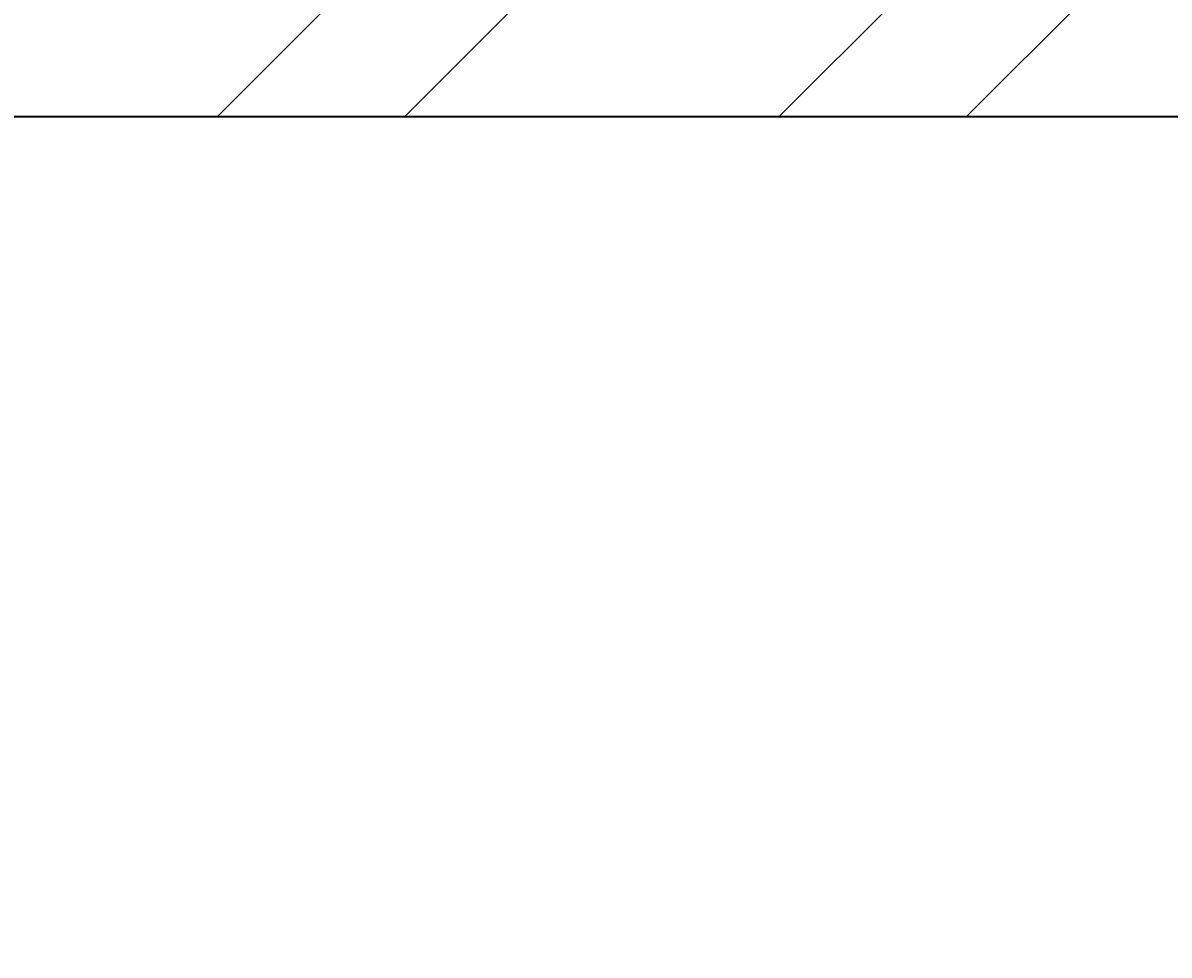
# Model space of a CAD drawing. Units: inches. Extents: x 1962 to 2771, y 1245 to 2660.
# Tile 70 of 114: x 2523 to 2551, y 2158 to 2180. Entities that reach past the tile are written whole.
import ezdxf

# ---------------------------------------------------------------- set-up
doc = ezdxf.new("R2010")
doc.units = ezdxf.units.IN
for name, color, linetype, lineweight in [('A-ANNO-DIMS', 2, 'Continuous', 18), ('A-WALL', 7, 'Continuous', 35), ('A-WALL-PATT', 252, 'Continuous', 13)]:
    doc.layers.add(name, color=color, linetype=linetype, lineweight=lineweight)
doc.styles.get("Standard").update_dxf_attribs({"font": 'arial.ttf'})
doc.dimstyles.get("Standard").update_dxf_attribs({"dimtxt": 0.18, "dimasz": 0.18, "dimexe": 0.18, "dimexo": 0.0625, "dimgap": 0.09, "dimtad": 0, "dimtih": 1, "dimtoh": 1, "dimdec": 4, "dimzin": 0, "dimdsep": 46, "dimtxsty": 'Standard', "dimcen": 0.09, "dimadec": 0, "dimazin": 0, "dimtfac": 1, "dimtdec": 4, "dimtofl": 0, "dimtmove": 0, "dimatfit": 3, "dimfxl": 1, "dimtolj": 1, "dimtzin": 0, "dimarcsym": 0})

# ---------------------------------------------------------------- blocks, each defined once
blk = doc.blocks.new('*D40')
at = {"layer": 'A-ANNO-DIMS', "color": 0, "lineweight": -2, "transparency": 16777216}
for p, q in [((2072.02, 2033.906), (2072.02, 2583.474)), ((2660.807, 2524.406), (2660.807, 2583.474)), ((2072.2, 2583.294), (2366.02, 2583.294)), ((2660.627, 2583.294), (2366.808, 2583.294))]:
    blk.add_line(p, q, dxfattribs=at)
at = {"layer": 'A-ANNO-DIMS', "color": 0, "transparency": 16777216}
for points in [[(2072.2, 2583.324), (2072.2, 2583.264), (2072.02, 2583.294)], [(2660.627, 2583.324), (2660.627, 2583.264), (2660.807, 2583.294)]]:
    blk.add_solid(points, dxfattribs=at)
at = {"layer": 'Defpoints', "color": 0, "transparency": 16777216}
for p in [(2660.807, 2583.294), (2660.807, 2524.344), (2072.02, 2033.844)]:
    blk.add_point(p, dxfattribs=at)
at = {"layer": 'A-ANNO-DIMS', "color": 0, "transparency": 16777216, "insert": (2366.414, 2583.294), "char_height": 0.18, "attachment_point": 5}
blk.add_mtext('\\A1;588.8', dxfattribs=at)

msp = doc.modelspace()

# ---------------------------------------------------------------- hatches: boundary and pattern name
at = {"layer": 'A-WALL-PATT'}
h = msp.add_hatch(dxfattribs=at)
h.set_pattern_fill('ANSI32', color=256)
h.paths.add_polyline_path([(2090.8074, 2467.3437), (2141.6481, 2467.3437), (2141.6481, 2469.5937), (2141.6481, 2471.8437), (2086.3074, 2471.8437), (2086.3074, 2422.5333), (2090.8074, 2422.5333)])
h.paths.add_polyline_path([(2282.7664, 2471.8437), (2204.8982, 2471.8437), (2204.8982, 2467.3437), (2234.8074, 2467.3437), (2234.8074, 2311.3437), (2228.7492, 2311.3437), (2228.7492, 2306.8437), (2234.8074, 2306.8437), (2331.9227, 2306.8437), (2331.9227, 2309.0937), (2331.9227, 2311.3437), (2239.3074, 2311.3437), (2239.3074, 2467.3437), (2282.7664, 2467.3437), (2282.7664, 2469.5937)])
h.paths.add_polyline_path([(2471.4531, 2519.8437), (2552.011, 2519.8437), (2564.3996, 2519.8437), (2564.3996, 2511.1389), (2568.8996, 2511.1389), (2568.8996, 2524.3437), (2466.9531, 2524.3437), (2466.9531, 2471.8437), (2450.0749, 2471.8437), (2446.4672, 2471.8437), (2446.4672, 2467.3437), (2450.0749, 2467.3437), (2475.9988, 2467.3437), (2475.9988, 2469.5937), (2475.9988, 2471.8437), (2471.4531, 2471.8437)])
h.paths.add_polyline_path([(2575.2231, 2469.5937), (2575.2231, 2471.8437), (2568.8996, 2471.8437), (2568.8996, 2487.1389), (2564.3996, 2487.1389), (2564.3996, 2471.8437), (2556.511, 2471.8437), (2499.2904, 2471.8437), (2499.2904, 2467.3437), (2507.8074, 2467.3437), (2507.8074, 2311.3437), (2414.863, 2311.3437), (2414.863, 2306.8437), (2512.3074, 2306.8437), (2517.0114, 2306.8437), (2517.0114, 2309.0937), (2517.0114, 2311.3437), (2512.3074, 2311.3437), (2512.3074, 2467.3437), (2575.2231, 2467.3437)])
h.paths.add_polyline_path([(2660.8074, 2471.8437), (2600.9602, 2471.8437), (2600.9602, 2467.3437), (2656.3074, 2467.3437), (2656.3074, 2432.5704), (2660.8074, 2432.5704)])
h.paths.add_polyline_path([(2660.8074, 2372.5704), (2656.3074, 2372.5704), (2656.3074, 2311.3437), (2600.276, 2311.3437), (2600.276, 2309.0937), (2600.276, 2306.8437), (2656.3074, 2306.8437), (2656.3074, 2296.2593), (2660.8074, 2296.2593)])
h.paths.add_polyline_path([(2572.3074, 2306.8437), (2577.1385, 2306.8437), (2577.1385, 2311.3437), (2551.082, 2311.3437), (2551.082, 2306.8437), (2567.8074, 2306.8437), (2567.8074, 2258.8437), (2540.0574, 2258.8437), (2540.0574, 2256.5937), (2540.0574, 2254.3437), (2567.8074, 2254.3437), (2656.3074, 2254.3437), (2656.3074, 2236.9085), (2660.8074, 2236.9085), (2660.8074, 2272.2593), (2656.3074, 2272.2593), (2656.3074, 2258.8437), (2572.3074, 2258.8437)])
h.paths.add_polyline_path([(2512.3074, 2254.3437), (2518.8716, 2254.3437), (2518.8716, 2256.5937), (2518.8716, 2258.8437), (2507.8074, 2258.8437), (2507.8074, 2177.8437), (2567.8074, 2177.8437), (2567.8074, 2172.9628), (2572.3074, 2172.9628), (2572.3074, 2177.8437), (2656.3074, 2177.8437), (2656.3074, 2166.4846), (2660.8074, 2166.4846), (2660.8074, 2200.9085), (2656.3074, 2200.9085), (2656.3074, 2182.3437), (2512.3074, 2182.3437)])
h.paths.add_polyline_path([(2656.3074, 2129.8437), (2572.3074, 2129.8437), (2572.3074, 2150.3044), (2570.0574, 2150.3044), (2567.8074, 2150.3044), (2567.8074, 2129.8437), (2507.8074, 2129.8437), (2507.8074, 2116.3027), (2510.0574, 2116.3027), (2512.3074, 2116.3027), (2512.3074, 2125.3437), (2567.8074, 2125.3437), (2572.3074, 2125.3437), (2656.3074, 2125.3437)])
h.paths.add_polyline_path([(2090.8074, 2362.5333), (2086.3074, 2362.5333), (2086.3074, 2298.6242), (2090.8074, 2298.6242), (2090.8074, 2306.8437), (2174.8074, 2306.8437), (2174.8074, 2286.4178), (2179.3074, 2286.4178), (2179.3074, 2306.8437), (2192.8641, 2306.8437), (2192.8641, 2309.0937), (2192.8641, 2311.3437), (2090.8074, 2311.3437)])
h.paths.add_polyline_path([(2209.156, 2258.8437), (2179.3074, 2258.8437), (2179.3074, 2263.2236), (2177.0574, 2263.2236), (2174.8074, 2263.2236), (2174.8074, 2258.8437), (2090.8074, 2258.8437), (2090.8074, 2274.6242), (2086.3074, 2274.6242), (2086.3074, 2238.2967), (2088.5574, 2238.2967), (2090.8074, 2238.2967), (2090.8074, 2254.3437), (2209.156, 2254.3437)])
h.paths.add_polyline_path([(2090.8074, 2177.8437), (2234.8074, 2177.8437), (2234.8074, 2173.1428), (2239.3074, 2173.1428), (2239.3074, 2258.8437), (2230.8442, 2258.8437), (2230.8442, 2256.5937), (2230.8442, 2254.3437), (2234.8074, 2254.3437), (2234.8074, 2182.3437), (2090.8074, 2182.3437), (2090.8074, 2202.2967), (2086.3074, 2202.2967), (2086.3074, 2140.0389), (2090.8074, 2140.0389)])
h.paths.add_polyline_path([(2090.8074, 2080.0389), (2086.3074, 2080.0389), (2086.3074, 2033.8437), (2090.8074, 2033.8437)], flags=17)
h.paths.add_polyline_path([(2244.9405, 2033.8437), (2239.3074, 2033.8437), (2239.3074, 2142.0665), (2237.2592, 2142.0665), (2234.8074, 2142.0665), (2234.8074, 2033.8437), (2090.8074, 2033.8437), (2076.5204, 2033.8437), (2072.0204, 2033.8437), (2072.0204, 2000.4493), (2076.5204, 2000.4493), (2076.5204, 2029.3437), (2090.8074, 2029.3437), (2244.9405, 2029.3437), (2244.9405, 2031.5937)])
h.paths.add_polyline_path([(2234.8074, 1933.3437), (2076.5204, 1933.3437), (2076.5204, 1952.4493), (2074.2704, 1952.4493), (2072.0204, 1952.4493), (2072.0204, 1933.3437), (2072.0204, 1928.8437), (2234.8074, 1928.8437)])
h.paths.add_polyline_path([(2090.8074, 1928.8437), (2086.3074, 1928.8437), (2086.3074, 1906.5013), (2090.8074, 1906.5013)])
h.paths.add_polyline_path([(2090.8074, 1846.5013), (2086.3074, 1846.5013), (2086.3074, 1769.9917), (2088.5574, 1769.9917), (2090.8074, 1769.9917), (2090.8074, 1780.3437), (2234.8074, 1780.3437), (2234.8074, 1708.3437), (2230.3764, 1708.3437), (2230.3764, 1703.8437), (2239.3074, 1703.8437), (2239.3074, 1792.6669), (2237.0574, 1792.6669), (2234.8074, 1792.6669), (2234.8074, 1784.8437), (2090.8074, 1784.8437)])
h.paths.add_polyline_path([(2239.3074, 1928.8437), (2244.9405, 1928.8437), (2244.9405, 1931.0937), (2244.9405, 1933.3437), (2234.8074, 1933.3437), (2234.8074, 1928.8437), (2234.8074, 1825.5949), (2239.3074, 1825.5949)])
h.paths.add_polyline_path([(2148.0425, 1649.0937), (2148.0425, 1651.3437), (2090.8074, 1651.3437), (2090.8074, 1646.8437), (2148.0425, 1646.8437)], flags=0)
h.paths.add_polyline_path([(2207.5601, 1708.3437), (2090.8074, 1708.3437), (2090.8074, 1703.8437), (2174.8074, 1703.8437), (2174.8074, 1651.3437), (2170.4457, 1651.3437), (2170.4457, 1646.8437), (2195.9924, 1646.8437), (2195.9924, 1649.0937), (2195.9924, 1651.3437), (2179.3074, 1651.3437), (2179.3074, 1703.8437), (2207.5601, 1703.8437), (2207.5601, 1706.0937)])
h.paths.add_polyline_path([(2090.8074, 1733.9917), (2086.3074, 1733.9917), (2086.3074, 1696.1032), (2088.5574, 1696.1032), (2090.8074, 1696.1032)])
h.paths.add_polyline_path([(2090.8074, 1672.1032), (2086.3074, 1672.1032), (2086.3074, 1600.3335), (2090.8074, 1600.3335)])
h.paths.add_polyline_path([(2090.8074, 1540.3335), (2086.3074, 1540.3335), (2086.3074, 1486.3437), (2139.6766, 1486.3437), (2139.6766, 1490.8437), (2090.8074, 1490.8437)])
h.paths.add_polyline_path([(2302.3876, 1490.8437), (2239.3074, 1490.8437), (2239.3074, 1646.8437), (2335.9994, 1646.8437), (2335.9994, 1651.3437), (2229.884, 1651.3437), (2229.884, 1646.8437), (2234.8074, 1646.8437), (2234.8074, 1490.8437), (2202.7103, 1490.8437), (2202.7103, 1488.5937), (2202.7103, 1486.3437), (2275.0699, 1486.3437), (2275.0699, 1475.772), (2279.5699, 1475.772), (2279.5699, 1486.3437), (2302.3876, 1486.3437)])
h.paths.add_polyline_path([(2279.5699, 1451.772), (2275.0699, 1451.772), (2275.0699, 1438.3437), (2174.8074, 1438.3437), (2174.8074, 1486.3437), (2179.7922, 1486.3437), (2179.7922, 1490.8437), (2163.3585, 1490.8437), (2163.3585, 1488.5937), (2163.3585, 1486.3437), (2170.3074, 1486.3437), (2170.3074, 1433.8437), (2279.5699, 1433.8437)])
h.paths.add_polyline_path([(2427.2363, 1490.8437), (2375.8074, 1490.8437), (2375.8074, 1646.8437), (2381.6401, 1646.8437), (2381.6401, 1651.3437), (2365.887, 1651.3437), (2365.887, 1649.0937), (2365.887, 1646.8437), (2371.3074, 1646.8437), (2371.3074, 1490.8437), (2327.5627, 1490.8437), (2327.5627, 1488.5937), (2327.5627, 1486.3437), (2371.3074, 1486.3437), (2371.3074, 1433.8437), (2375.8074, 1433.8437), (2375.8074, 1486.3437), (2427.2363, 1486.3437)])
h.paths.add_polyline_path([(2512.3074, 1646.8437), (2519.4351, 1646.8437), (2519.4351, 1649.0937), (2519.4351, 1651.3437), (2507.8074, 1651.3437), (2416.0063, 1651.3437), (2416.0063, 1649.0937), (2416.0063, 1646.8437), (2507.8074, 1646.8437), (2507.8074, 1490.8437), (2497.0532, 1490.8437), (2497.0532, 1488.5937), (2497.0532, 1486.3437), (2574.9344, 1486.3437), (2574.9344, 1476.0181), (2579.4344, 1476.0181), (2579.4344, 1486.3437), (2584.4872, 1486.3437), (2584.3074, 1490.8437), (2512.3074, 1490.8437)])
h.paths.add_polyline_path([(2470.5091, 1486.3437), (2473.9767, 1486.3437), (2473.9767, 1490.8437), (2449.6605, 1490.8437), (2449.6605, 1488.5937), (2449.6605, 1486.3437), (2466.0091, 1486.3437), (2466.0091, 1433.8437), (2470.5091, 1433.8437), (2579.4344, 1433.8437), (2579.4344, 1452.0181), (2574.9344, 1452.0181), (2574.9344, 1438.3437), (2554.5091, 1438.3437), (2470.5091, 1438.3437)])
h.paths.add_polyline_path([(2656.3074, 1490.8437), (2611.86, 1490.8437), (2611.86, 1486.3437), (2656.3074, 1486.3437)])
h.paths.add_polyline_path([(2660.8074, 1532.7007), (2658.5574, 1532.7007), (2656.3074, 1532.7007), (2656.3074, 1486.3437), (2660.8074, 1486.3437)])
h.paths.add_polyline_path([(2660.8074, 1664.9663), (2656.3074, 1664.9663), (2656.3074, 1651.3437), (2602.2313, 1651.3437), (2602.2313, 1646.8437), (2656.3074, 1646.8437), (2656.3074, 1592.7007), (2660.8074, 1592.7007)])
h.paths.add_polyline_path([(2660.8074, 1724.5221), (2656.3074, 1724.5221), (2656.3074, 1703.8437), (2542.4725, 1703.8437), (2542.4725, 1699.3437), (2567.8074, 1699.3437), (2567.8074, 1651.3437), (2552.7766, 1651.3437), (2552.7766, 1649.0937), (2552.7766, 1646.8437), (2577.2878, 1646.8437), (2577.2878, 1649.0937), (2577.2878, 1651.3437), (2572.3074, 1651.3437), (2572.3074, 1699.3437), (2656.3074, 1699.3437), (2656.3074, 1688.9663), (2660.8074, 1688.9663)])
h.paths.add_polyline_path([(2660.8074, 1880.6524), (2656.3074, 1880.6524), (2656.3074, 1832.8437), (2512.3074, 1832.8437), (2512.3074, 1837.8959), (2507.8074, 1837.8959), (2507.8074, 1828.3437), (2567.8074, 1828.3437), (2567.8074, 1804.3437), (2572.3074, 1804.3437), (2572.3074, 1828.3437), (2656.3074, 1828.3437), (2656.3074, 1818.6778), (2660.8074, 1818.6778)])
h.paths.add_polyline_path([(2660.8074, 1794.6778), (2656.3074, 1794.6778), (2656.3074, 1780.3437), (2572.3074, 1780.3437), (2572.3074, 1783.0303), (2570.0574, 1783.0303), (2567.8074, 1783.0303), (2567.8074, 1780.3437), (2507.8074, 1780.3437), (2507.8074, 1699.3437), (2517.8858, 1699.3437), (2517.8858, 1701.5937), (2517.8858, 1703.8437), (2512.3074, 1703.8437), (2512.3074, 1775.8437), (2656.3074, 1775.8437), (2656.3074, 1760.5221), (2660.8074, 1760.5221)])
h.paths.add_polyline_path([(2660.8074, 1981.3437), (2660.8074, 2020.2808), (2658.5574, 2020.2808), (2656.3074, 2020.2808), (2656.3074, 1981.3437), (2512.3074, 1981.3437), (2512.3074, 2086.6996), (2507.8074, 2086.6996), (2507.8074, 1981.3437), (2375.8074, 1981.3437), (2375.8074, 1986.8505), (2373.5574, 1986.8505), (2371.3074, 1986.8505), (2371.3074, 1973.2607), (2375.8074, 1973.2607), (2375.8074, 1976.8437), (2507.8074, 1976.8437), (2507.8074, 1865.4281), (2510.0574, 1865.4281), (2512.3074, 1865.4281), (2512.3074, 1976.8437), (2660.8074, 1976.8437)])
h.paths.add_polyline_path([(2375.8074, 1940.297), (2373.5574, 1940.297), (2371.3074, 1940.297), (2371.3074, 1933.3437), (2278.4434, 1933.3437), (2278.4434, 1928.8437), (2371.3074, 1928.8437), (2371.3074, 1651.3437), (2375.8074, 1651.3437)])
h.paths.add_polyline_path([(2660.8074, 1976.8437), (2656.3074, 1976.8437), (2656.3074, 1940.6524), (2660.8074, 1940.6524)], flags=17)
h.paths.add_polyline_path([(2660.8074, 2142.4846), (2656.3074, 2142.4846), (2656.3074, 2080.2808), (2660.8074, 2080.2808)])
h.paths.add_polyline_path([(2381.4189, 2311.3437), (2375.8074, 2311.3437), (2375.8074, 2467.3437), (2424.7242, 2467.3437), (2424.7242, 2469.5937), (2424.7242, 2471.8437), (2375.8074, 2471.8437), (2375.8074, 2524.3437), (2371.3074, 2524.3437), (2371.3074, 2471.8437), (2307.2097, 2471.8437), (2307.2097, 2467.3437), (2371.3074, 2467.3437), (2371.3074, 2311.3437), (2366.8901, 2311.3437), (2366.8901, 2306.8437), (2371.3074, 2306.8437), (2371.3074, 2033.8437), (2279.6589, 2033.8437), (2279.6589, 2029.3437), (2371.3074, 2029.3437), (2371.3074, 2014.2598), (2375.8074, 2014.2598), (2375.8074, 2306.8437), (2381.4189, 2306.8437)])
h.paths.add_polyline_path([(2263.3074, 2524.3437), (2170.3074, 2524.3437), (2170.3074, 2519.8437), (2170.3074, 2471.8437), (2165.0312, 2471.8437), (2165.0312, 2467.3437), (2179.6721, 2467.3437), (2179.6721, 2469.5161), (2179.6721, 2471.8437), (2174.8074, 2471.8437), (2174.8074, 2519.8437), (2258.8074, 2519.8437), (2258.8074, 2511.6436), (2263.3074, 2511.6436)])
h.paths.add_polyline_path([(2245.0232, 1361.4123), (2492.9468, 1361.4123), (2492.9468, 1398.505), (2245.0232, 1398.505)], flags=9)
h.paths.add_polyline_path([(2388.1434, 2086.6936), (2425.0704, 2086.6936), (2425.0704, 2105.3509), (2388.1434, 2105.3509)], flags=9)
h.paths.add_polyline_path([(2404.922, 2242.6744), (2445.7337, 2242.6744), (2445.7337, 2261.3318), (2404.922, 2261.3318)], flags=9)
h.paths.add_polyline_path([(2269.4107, 2156.7935), (2306.3378, 2156.7935), (2306.3378, 2175.4508), (2269.4107, 2175.4508)], flags=9)
h.paths.add_polyline_path([(2269.3277, 2233.4343), (2306.2547, 2233.4343), (2306.2547, 2252.0917), (2269.3277, 2252.0917)], flags=9)
h.paths.add_polyline_path([(2431.6052, 2320.6922), (2470.4456, 2320.6922), (2470.4456, 2339.3495), (2431.6052, 2339.3495)], flags=25)
h.paths.add_polyline_path([(2249.6902, 2315.7608), (2288.5306, 2315.7608), (2288.5306, 2334.4182), (2249.6902, 2334.4182)], flags=25)
h.paths.add_polyline_path([(2096.9301, 2314.3181), (2135.7704, 2314.3181), (2135.7704, 2332.9755), (2096.9301, 2332.9755)], flags=25)
h.paths.add_polyline_path([(2134.3475, 2285.7089), (2161.4655, 2285.7089), (2161.4655, 2304.3662), (2134.3475, 2304.3662)], flags=9)
h.paths.add_polyline_path([(2126.5155, 2209.4076), (2159.9227, 2209.4076), (2159.9227, 2228.065), (2126.5155, 2228.065)], flags=25)
h.paths.add_polyline_path([(2110.5753, 2141.5299), (2149.4157, 2141.5299), (2149.4157, 2160.1872), (2110.5753, 2160.1872)], flags=25)
h.paths.add_polyline_path([(2249.8618, 1968.3317), (2286.3966, 1968.3317), (2286.3966, 1986.989), (2249.8618, 1986.989)], flags=9)
h.paths.add_polyline_path([(2395.9507, 1777.0051), (2436.7624, 1777.0051), (2436.7624, 1795.6625), (2395.9507, 1795.6625)], flags=9)
h.paths.add_polyline_path([(2398.5259, 1888.5651), (2435.0062, 1888.5651), (2435.0062, 1907.2224), (2398.5259, 1907.2224)], flags=25)
h.paths.add_polyline_path([(2259.3506, 1728.3559), (2296.2776, 1728.3559), (2296.2776, 1747.0132), (2259.3506, 1747.0132)], flags=9)
h.paths.add_polyline_path([(2271.3698, 1845.268), (2308.2968, 1845.268), (2308.2968, 1863.9253), (2271.3698, 1863.9253)], flags=9)
h.paths.add_polyline_path([(2120.9355, 1786.3027), (2159.7759, 1786.3027), (2159.7759, 1804.9601), (2120.9355, 1804.9601)], flags=25)
h.paths.add_polyline_path([(2121.3164, 1732.1043), (2154.7236, 1732.1043), (2154.7236, 1750.7616), (2121.3164, 1750.7616)], flags=25)
h.paths.add_polyline_path([(2118.3706, 1678.8997), (2147.5282, 1678.8997), (2147.5282, 1697.557), (2118.3706, 1697.557)], flags=25)
h.paths.add_polyline_path([(2385.9227, 1493.557), (2424.763, 1493.557), (2424.763, 1512.2143), (2385.9227, 1512.2143)], flags=25)
h.paths.add_polyline_path([(2248.7058, 1500.0256), (2287.5462, 1500.0256), (2287.5462, 1518.6829), (2248.7058, 1518.6829)], flags=25)
h.paths.add_polyline_path([(2104.1669, 1617.3771), (2143.0073, 1617.3771), (2143.0073, 1636.0344), (2104.1669, 1636.0344)], flags=9)
h.paths.add_polyline_path([(2096.0714, 1447.8824), (2137.3845, 1447.8824), (2137.3845, 1458.1859), (2096.0714, 1458.1859)], flags=9)
h.paths.add_polyline_path([(2180.6114, 1440.325), (2209.7689, 1440.325), (2209.7689, 1458.9823), (2180.6114, 1458.9823)], flags=25)
h.paths.add_polyline_path([(2316.1698, 1447.9637), (2357.4829, 1447.9637), (2357.4829, 1458.2673), (2316.1698, 1458.2673)], flags=9)
h.paths.add_polyline_path([(2397.6187, 1447.9637), (2438.9318, 1447.9637), (2438.9318, 1458.2673), (2397.6187, 1458.2673)], flags=9)
h.paths.add_polyline_path([(2473.0778, 1439.5953), (2502.2354, 1439.5953), (2502.2354, 1458.2527), (2473.0778, 1458.2527)], flags=25)
h.paths.add_polyline_path([(2589.7027, 1447.8819), (2631.0158, 1447.8819), (2631.0158, 1458.1855), (2589.7027, 1458.1855)], flags=9)
h.paths.add_polyline_path([(2522.4009, 1497.5285), (2561.2413, 1497.5285), (2561.2413, 1516.1859), (2522.4009, 1516.1859)], flags=25)
h.paths.add_polyline_path([(2579.6565, 1671.3482), (2608.8141, 1671.3482), (2608.8141, 1690.0056), (2579.6565, 1690.0056)], flags=25)
h.paths.add_polyline_path([(2544.7038, 1725.5064), (2578.1111, 1725.5064), (2578.1111, 1744.1637), (2544.7038, 1744.1637)], flags=25)
h.paths.add_polyline_path([(2578.1191, 1807.472), (2607.2766, 1807.472), (2607.2766, 1826.1293), (2578.1191, 1826.1293)], flags=25)
h.paths.add_polyline_path([(2595.0614, 1835.1839), (2633.9018, 1835.1839), (2633.9018, 1853.8413), (2595.0614, 1853.8413)], flags=25)
h.paths.add_polyline_path([(2567.0097, 2097.7035), (2605.8501, 2097.7035), (2605.8501, 2116.3609), (2567.0097, 2116.3609)], flags=9)
h.paths.add_polyline_path([(2586.644, 2134.6454), (2615.8015, 2134.6454), (2615.8015, 2153.3027), (2586.644, 2153.3027)], flags=9)
h.paths.add_polyline_path([(2544.6185, 2212.6783), (2578.0258, 2212.6783), (2578.0258, 2231.3356), (2544.6185, 2231.3356)], flags=25)
h.paths.add_polyline_path([(2577.0273, 2256.9023), (2606.1849, 2256.9023), (2606.1849, 2275.5597), (2577.0273, 2275.5597)], flags=24)
h.paths.add_polyline_path([(2605.2683, 2315.2821), (2644.1087, 2315.2821), (2644.1087, 2333.9395), (2605.2683, 2333.9395)], flags=25)
h.paths.add_polyline_path([(2583.1244, 2496.1815), (2624.4375, 2496.1815), (2624.4375, 2506.4851), (2583.1244, 2506.4851)], flags=9)
h.paths.add_polyline_path([(2474.761, 2497.0823), (2503.9185, 2497.0823), (2503.9185, 2515.7397), (2474.761, 2515.7397)], flags=25)
h.paths.add_polyline_path([(2387.5787, 2494.2563), (2428.902, 2494.2563), (2428.902, 2504.5598), (2387.5787, 2504.5598)], flags=9)
h.paths.add_polyline_path([(2300.1657, 2500.1564), (2341.4788, 2500.1564), (2341.4788, 2510.46), (2300.1657, 2510.46)], flags=25)
h.paths.add_polyline_path([(2176.8589, 2497.5843), (2206.0165, 2497.5843), (2206.0165, 2516.2416), (2176.8589, 2516.2416)], flags=25)
h.paths.add_polyline_path([(2097.4668, 2494.9762), (2138.7799, 2494.9762), (2138.7799, 2505.2798), (2097.4668, 2505.2798)], flags=9)

# ---------------------------------------------------------------- linework, layer by layer
at = {"layer": 'A-WALL'}
msp.add_line((2567.8074, 2177.8437), (2507.8074, 2177.8437), dxfattribs=at)

# ---------------------------------------------------------------- dimensions: what is measured, and where the dimension line sits
at = {"layer": 'A-ANNO-DIMS'}
dim = msp.add_linear_dim(base=(2660.8074, 2583.2937), p1=(2072.0204, 2033.8437), p2=(2660.8074, 2524.3437), dimstyle='Standard', override={"dimdec": 1, "dimlfac": 1, "dimrnd": 0, "dimzin": 0, "dimdsep": 46, "dimlunit": 2}, dxfattribs=at)
dim.commit()
dim.dimension.update_dxf_attribs({"geometry": '*D40', "text_midpoint": (2366.4139, 2583.2937)})

doc.saveas('drawing.dxf')
